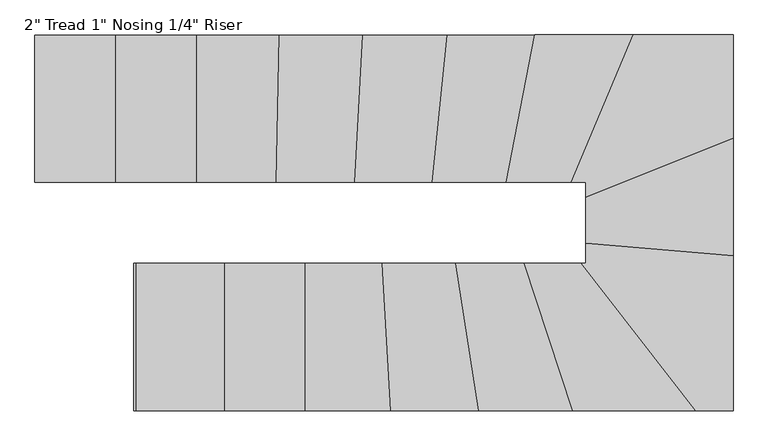
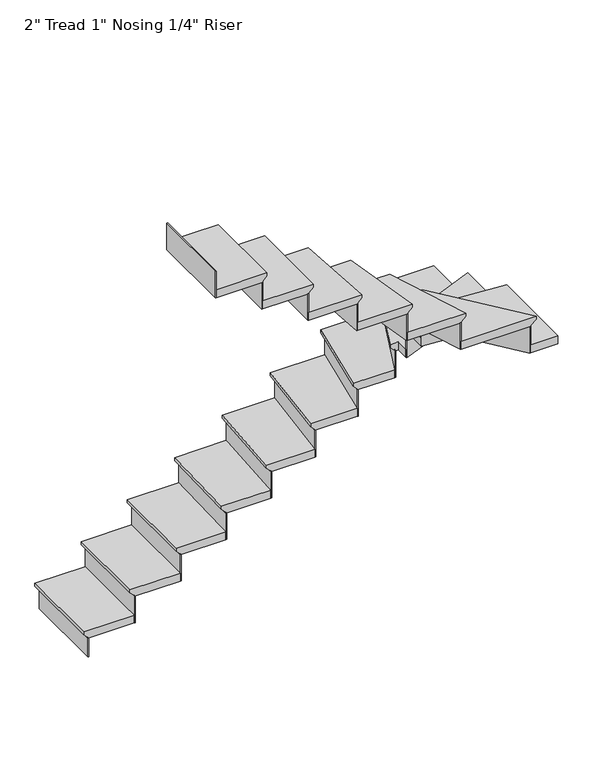
"""IFC4 building model written with IfcOpenShell, lengths in millimetres: stair flight geometry."""

from ifc_helpers import new_model, si_unit, origin, place, context, project, spatial, faceted_brep, source, transform, mapped, element, save


def stair_flight_4e66bfb9(model_context):
    return source(origin(), model_context, "Body", "Brep", [
        faceted_brep([(838.4202681, 2693.877558, 3520.0166667), (838.4202681, 2693.877558, 3539.0666667), (838.4202681, 3202.4524989, 3539.0666667), (838.4202681, 3202.4524989, 3520.0166667), (863.8202681, 2693.877558, 3494.6166667), (863.8202681, 3202.4524989, 3494.6166667), (1143.2202681, 2693.877558, 3539.0666667), (1143.2202681, 3202.4524989, 3539.0666667), (863.8202681, 3202.4524989, 3488.2666667), (1143.2202681, 3202.4524989, 3488.2666667), (1143.2202681, 2693.877558, 3488.2666667), (863.8202681, 2693.877558, 3488.2666667)], [[[0, 1, 2, 3]], [[4, 0, 3, 5]], [[2, 1, 6, 7]], [[8, 9, 10, 11]], [[2, 7, 9, 8, 5, 3]], [[8, 11, 4, 5]], [[6, 1, 0, 4, 11, 10]], [[7, 6, 10, 9]]]),
        faceted_brep([(863.8202681, 2693.877558, 3488.2666667), (863.8202681, 2693.877558, 3369.7333333), (870.1702681, 2693.877558, 3369.7333333), (870.1702681, 2693.877558, 3488.2666667), (863.8202681, 3202.4524989, 3488.2666667), (870.1702681, 3202.4524989, 3488.2666667), (870.1702681, 3202.4524989, 3369.7333333), (863.8202681, 3202.4524989, 3369.7333333)], [[[0, 1, 2, 3]], [[4, 5, 6, 7]], [[1, 0, 4, 7]], [[2, 1, 7, 6]], [[3, 2, 6, 5]], [[0, 3, 5, 4]]]),
        faceted_brep([(1143.2202681, 2693.877558, 3657.6), (1143.2202681, 2693.877558, 3488.2666667), (1149.5702681, 2693.877558, 3488.2666667), (1149.5702681, 2693.877558, 3657.6), (1143.2202681, 3202.4524989, 3657.6), (1149.5702681, 3202.4524989, 3657.6), (1149.5702681, 3202.4524989, 3488.2666667), (1143.2202681, 3202.4524989, 3488.2666667)], [[[0, 1, 2, 3]], [[4, 5, 6, 7]], [[1, 0, 4, 7]], [[2, 1, 7, 6]], [[3, 2, 6, 5]], [[0, 3, 5, 4]]]),
        faceted_brep([(1117.8202681, 3202.4524989, 3708.4), (1117.8202681, 2693.877558, 3708.4), (1422.6202681, 2693.877558, 3708.4), (1422.6202681, 3202.4524989, 3708.4), (1143.2202681, 3202.4524989, 3657.6), (1422.6202681, 3202.4524989, 3657.6), (1422.6202681, 2693.877558, 3657.6), (1143.2202681, 2693.877558, 3657.6), (1143.2202681, 3202.4524989, 3663.95), (1117.8202681, 3202.4524989, 3689.35), (1143.2202681, 2693.877558, 3663.95), (1117.8202681, 2693.877558, 3689.35)], [[[0, 1, 2, 3]], [[4, 5, 6, 7]], [[0, 3, 5, 4, 8, 9]], [[4, 7, 10, 8]], [[2, 1, 11, 10, 7, 6]], [[3, 2, 6, 5]], [[11, 1, 0, 9]], [[10, 11, 9, 8]]]),
        faceted_brep([(1422.6202681, 2693.877558, 3826.9333333), (1422.6202681, 2693.877558, 3657.6), (1428.9702681, 2693.877558, 3657.6), (1428.9702681, 2693.877558, 3826.9333333), (1422.6202681, 3202.4524989, 3826.9333333), (1428.9702681, 3202.4524989, 3826.9333333), (1428.9702681, 3202.4524989, 3657.6), (1422.6202681, 3202.4524989, 3657.6)], [[[0, 1, 2, 3]], [[4, 5, 6, 7]], [[1, 0, 4, 7]], [[2, 1, 7, 6]], [[3, 2, 6, 5]], [[0, 3, 5, 4]]]),
        faceted_brep([(1397.2202681, 3202.4524989, 3877.7333333), (1397.2202681, 2693.877558, 3877.7333333), (1696.6553711, 2693.877558, 3877.7333333), (1707.3964935, 3202.4524989, 3877.7333333), (1422.6202681, 3202.4524989, 3826.9333333), (1707.3964935, 3202.4524989, 3826.9333333), (1696.6553711, 2693.877558, 3826.9333333), (1422.6202681, 2693.877558, 3826.9333333), (1422.6202681, 3202.4524989, 3833.2833333), (1397.2202681, 3202.4524989, 3858.6833333), (1422.6202681, 2693.877558, 3833.2833333), (1397.2202681, 2693.877558, 3858.6833333)], [[[0, 1, 2, 3]], [[4, 5, 6, 7]], [[0, 3, 5, 4, 8, 9]], [[4, 7, 10, 8]], [[2, 1, 11, 10, 7, 6]], [[3, 2, 6, 5]], [[11, 1, 0, 9]], [[10, 11, 9, 8]]]),
        faceted_brep([(1696.6553711, 2693.877558, 3996.2666667), (1696.6553711, 2693.877558, 3826.9333333), (1703.0067872, 2693.877558, 3826.9333333), (1703.0067872, 2693.877558, 3996.2666667), (1707.3964935, 3202.4524989, 3996.2666667), (1713.7479096, 3202.4524989, 3996.2666667), (1713.7479096, 3202.4524989, 3826.9333333), (1707.3964935, 3202.4524989, 3826.9333333)], [[[0, 1, 2, 3]], [[4, 5, 6, 7]], [[1, 0, 4, 7]], [[2, 1, 7, 6]], [[3, 2, 6, 5]], [[0, 3, 5, 4]]]),
        faceted_brep([(1681.9908293, 3202.4524989, 4047.0666667), (1671.2497068, 2693.877558, 4047.0666667), (1968.2389719, 2693.877558, 4047.0666667), (1994.6701229, 3202.4524989, 4047.0666667), (1707.3964935, 3202.4524989, 3996.2666667), (1994.6701229, 3202.4524989, 3996.2666667), (1968.2389719, 2693.877558, 3996.2666667), (1696.6553711, 2693.877558, 3996.2666667), (1707.3964935, 3202.4524989, 4002.6166667), (1681.9908293, 3202.4524989, 4028.0166667), (1696.6553711, 2693.877558, 4002.6166667), (1671.2497068, 2693.877558, 4028.0166667)], [[[0, 1, 2, 3]], [[4, 5, 6, 7]], [[0, 3, 5, 4, 8, 9]], [[4, 7, 10, 8]], [[2, 1, 11, 10, 7, 6]], [[3, 2, 6, 5]], [[11, 1, 0, 9]], [[10, 11, 9, 8]]]),
        faceted_brep([(1968.2389719, 2693.877558, 4165.6), (1968.2389719, 2693.877558, 3996.2666667), (1974.5975418, 2693.877558, 3996.2666667), (1974.5975418, 2693.877558, 4165.6), (1994.6701229, 3202.4524989, 4165.6), (2001.0286928, 3202.4524989, 4165.6), (2001.0286928, 3202.4524989, 3996.2666667), (1994.6701229, 3202.4524989, 3996.2666667)], [[[0, 1, 2, 3]], [[4, 5, 6, 7]], [[1, 0, 4, 7]], [[2, 1, 7, 6]], [[3, 2, 6, 5]], [[0, 3, 5, 4]]]),
        faceted_brep([(1969.2358436, 3202.4524989, 4216.4), (1942.8046925, 2693.877558, 4216.4), (2235.1931673, 2693.877558, 4216.4), (2286.7073051, 3202.4524989, 4216.4), (1994.6701229, 3202.4524989, 4165.6), (2286.7073051, 3202.4524989, 4165.6), (2235.1931673, 2693.877558, 4165.6), (1968.2389719, 2693.877558, 4165.6), (1994.6701229, 3202.4524989, 4171.95), (1969.2358436, 3202.4524989, 4197.35), (1968.2389719, 2693.877558, 4171.95), (1942.8046925, 2693.877558, 4197.35)], [[[0, 1, 2, 3]], [[4, 5, 6, 7]], [[0, 3, 5, 4, 8, 9]], [[4, 7, 10, 8]], [[2, 1, 11, 10, 7, 6]], [[3, 2, 6, 5]], [[11, 1, 0, 9]], [[10, 11, 9, 8]]]),
        faceted_brep([(2235.1931673, 2693.877558, 4334.9333333), (2235.1931673, 2693.877558, 4165.6), (2241.5756594, 2693.877558, 4165.6), (2241.5756594, 2693.877558, 4334.9333333), (2286.7073051, 3202.4524989, 4334.9333333), (2293.0897971, 3202.4524989, 4334.9333333), (2293.0897971, 3202.4524989, 4165.6), (2286.7073051, 3202.4524989, 4165.6)], [[[0, 1, 2, 3]], [[4, 5, 6, 7]], [[1, 0, 4, 7]], [[2, 1, 7, 6]], [[3, 2, 6, 5]], [[0, 3, 5, 4]]]),
        faceted_brep([(2261.1773369, 3202.4524989, 4385.7333333), (2209.6631992, 2693.877558, 4385.7333333), (2491.6737127, 2693.877558, 4385.7333333), (2589.7018996, 3202.4524989, 4385.7333333), (2286.7073051, 3202.4524989, 4334.9333333), (2589.7018996, 3202.4524989, 4334.9333333), (2491.6737127, 2693.877558, 4334.9333333), (2235.1931673, 2693.877558, 4334.9333333), (2286.7073051, 3202.4524989, 4341.2833333), (2261.1773369, 3202.4524989, 4366.6833333), (2235.1931673, 2693.877558, 4341.2833333), (2209.6631992, 2693.877558, 4366.6833333)], [[[0, 1, 2, 3]], [[4, 5, 6, 7]], [[0, 3, 5, 4, 8, 9]], [[4, 7, 10, 8]], [[2, 1, 11, 10, 7, 6]], [[3, 2, 6, 5]], [[11, 1, 0, 9]], [[10, 11, 9, 8]]]),
        faceted_brep([(2491.6737127, 2693.877558, 4504.2666667), (2491.6737127, 2693.877558, 4334.9333333), (2498.1405972, 2693.877558, 4334.9333333), (2498.1405972, 2693.877558, 4504.2666667), (2589.7018996, 3202.4524989, 4504.2666667), (2596.1687841, 3202.4524989, 4504.2666667), (2596.1687841, 3202.4524989, 4334.9333333), (2589.7018996, 3202.4524989, 4334.9333333)], [[[0, 1, 2, 3]], [[4, 5, 6, 7]], [[1, 0, 4, 7]], [[2, 1, 7, 6]], [[3, 2, 6, 5]], [[0, 3, 5, 4]]]),
        faceted_brep([(2563.8343615, 3202.4524989, 4555.0666667), (2465.8061746, 2693.877558, 4555.0666667), (2717.082711, 2693.877558, 4555.0666667), (2931.3822032, 3202.4524989, 4555.0666667), (2589.7018996, 3202.4524989, 4504.2666667), (2931.3822032, 3202.4524989, 4504.2666667), (2717.082711, 2693.877558, 4504.2666667), (2491.6737127, 2693.877558, 4504.2666667), (2589.7018996, 3202.4524989, 4510.6166667), (2563.8343615, 3202.4524989, 4536.0166667), (2491.6737127, 2693.877558, 4510.6166667), (2465.8061746, 2693.877558, 4536.0166667)], [[[0, 1, 2, 3]], [[4, 5, 6, 7]], [[0, 3, 5, 4, 8, 9]], [[4, 7, 10, 8]], [[2, 1, 11, 10, 7, 6]], [[3, 2, 6, 5]], [[11, 1, 0, 9]], [[10, 11, 9, 8]]]),
        faceted_brep([(2717.082711, 2693.877558, 4673.6), (2717.082711, 2693.877558, 4504.2666667), (2723.973426, 2693.877558, 4504.2666667), (2723.973426, 2693.877558, 4673.6), (2931.3822032, 3202.4524989, 4673.6), (2938.2729181, 3202.4524989, 4673.6), (2938.2729181, 3202.4524989, 4504.2666667), (2931.3822032, 3202.4524989, 4504.2666667)], [[[0, 1, 2, 3]], [[4, 5, 6, 7]], [[1, 0, 4, 7]], [[2, 1, 7, 6]], [[3, 2, 6, 5]], [[0, 3, 5, 4]]]),
        faceted_brep([(3247.982332, 2818.4435318, 4724.4), (3247.982332, 3202.4524989, 4724.4), (2903.8193433, 3202.4524989, 4724.4), (2689.5198512, 2693.877558, 4724.4), (2739.4073911, 2693.877558, 4724.4), (2739.4073911, 2614.5975609, 4724.4), (3247.982332, 3202.4524989, 4673.6), (3247.982332, 2818.4435318, 4673.6), (2739.4073911, 2614.5975609, 4673.6), (2739.4073911, 2693.877558, 4673.6), (2717.082711, 2693.877558, 4673.6), (2931.3822032, 3202.4524989, 4673.6), (2717.082711, 2693.877558, 4679.95), (2931.3822032, 3202.4524989, 4679.95), (2689.5198512, 2693.877558, 4705.35), (2903.8193433, 3202.4524989, 4705.35)], [[[0, 1, 2, 3, 4, 5]], [[6, 7, 8, 9, 10, 11]], [[1, 0, 7, 6]], [[11, 10, 12, 13]], [[5, 4, 9, 8]], [[0, 5, 8, 7]], [[14, 3, 2, 15]], [[12, 14, 15, 13]], [[4, 3, 14, 12, 10, 9]], [[2, 1, 6, 11, 13, 15]]]),
        faceted_brep([(2739.4073911, 2614.5975609, 4842.9333333), (2739.4073911, 2614.5975609, 4673.6), (2739.4073911, 2607.7564709, 4673.6), (2739.4073911, 2607.7564709, 4842.9333333), (3247.982332, 2818.4435318, 4842.9333333), (3247.982332, 2811.6024418, 4842.9333333), (3247.982332, 2811.6024418, 4673.6), (3247.982332, 2818.4435318, 4673.6)], [[[0, 1, 2, 3]], [[4, 5, 6, 7]], [[1, 0, 4, 7]], [[2, 1, 7, 6]], [[3, 2, 6, 5]], [[0, 3, 5, 4]]]),
        faceted_brep([(3247.982332, 2845.807892, 4893.7333333), (2739.4073911, 2641.9619211, 4893.7333333), (2739.4073911, 2458.7583414, 4893.7333333), (3247.982332, 2415.6151582, 4893.7333333), (3247.982332, 2818.4435318, 4842.9333333), (3247.982332, 2415.6151582, 4842.9333333), (2739.4073911, 2458.7583414, 4842.9333333), (2739.4073911, 2614.5975609, 4842.9333333), (3247.982332, 2818.4435318, 4849.2833333), (3247.982332, 2845.807892, 4874.6833333), (2739.4073911, 2614.5975609, 4849.2833333), (2739.4073911, 2641.9619211, 4874.6833333)], [[[0, 1, 2, 3]], [[4, 5, 6, 7]], [[0, 3, 5, 4, 8, 9]], [[4, 7, 10, 8]], [[2, 1, 11, 10, 7, 6]], [[3, 2, 6, 5]], [[11, 1, 0, 9]], [[10, 11, 9, 8]]]),
        faceted_brep([(2739.4073911, 2458.7583414, 5012.2666667), (2739.4073911, 2458.7583414, 4842.9333333), (2739.4073911, 2452.3855338, 4842.9333333), (2739.4073911, 2452.3855338, 5012.2666667), (3247.982332, 2415.6151582, 5012.2666667), (3247.982332, 2409.2423506, 5012.2666667), (3247.982332, 2409.2423506, 4842.9333333), (3247.982332, 2415.6151582, 4842.9333333)], [[[0, 1, 2, 3]], [[4, 5, 6, 7]], [[1, 0, 4, 7]], [[2, 1, 7, 6]], [[3, 2, 6, 5]], [[0, 3, 5, 4]]]),
        faceted_brep([(3085.5772675, 1905.9026171, 5063.0666667), (3247.982332, 1905.9026171, 5063.0666667), (3247.982332, 2441.1063885, 5063.0666667), (2739.4073911, 2484.2495716, 5063.0666667), (2739.4073911, 2414.477558, 5063.0666667), (2689.4386829, 2414.477558, 5063.0666667), (3247.982332, 1905.9026171, 5012.2666667), (3085.5772675, 1905.9026171, 5012.2666667), (2689.4386829, 2414.477558, 5012.2666667), (2739.4073911, 2414.477558, 5012.2666667), (2739.4073911, 2458.7583414, 5012.2666667), (3247.982332, 2415.6151582, 5012.2666667), (2739.4073911, 2458.7583414, 5018.6166667), (3247.982332, 2415.6151582, 5018.6166667), (2739.4073911, 2484.2495716, 5044.0166667), (3247.982332, 2441.1063885, 5044.0166667)], [[[0, 1, 2, 3, 4, 5]], [[6, 7, 8, 9, 10, 11]], [[1, 0, 7, 6]], [[11, 10, 12, 13]], [[4, 3, 14, 12, 10, 9]], [[5, 4, 9, 8]], [[0, 5, 8, 7]], [[14, 3, 2, 15]], [[12, 14, 15, 13]], [[2, 1, 6, 11, 13, 15]]]),
        faceted_brep([(2689.4386829, 2414.477558, 5181.6), (2689.4386829, 2414.477558, 5012.2666667), (2681.3896615, 2414.477558, 5012.2666667), (2681.3896615, 2414.477558, 5181.6), (3085.5772675, 1905.9026171, 5181.6), (3077.5282461, 1905.9026171, 5181.6), (3077.5282461, 1905.9026171, 5012.2666667), (3085.5772675, 1905.9026171, 5012.2666667)], [[[0, 1, 2, 3]], [[4, 5, 6, 7]], [[1, 0, 4, 7]], [[2, 1, 7, 6]], [[3, 2, 6, 5]], [[0, 3, 5, 4]]]),
        faceted_brep([(3117.7733531, 1905.9026171, 5232.4), (2721.6347685, 2414.477558, 5232.4), (2498.169104, 2414.477558, 5232.4), (2665.6971357, 1905.9026171, 5232.4), (3085.5772675, 1905.9026171, 5181.6), (2665.6971357, 1905.9026171, 5181.6), (2498.169104, 2414.477558, 5181.6), (2689.4386829, 2414.477558, 5181.6), (3085.5772675, 1905.9026171, 5187.95), (3117.7733531, 1905.9026171, 5213.35), (2689.4386829, 2414.477558, 5187.95), (2721.6347685, 2414.477558, 5213.35)], [[[0, 1, 2, 3]], [[4, 5, 6, 7]], [[0, 3, 5, 4, 8, 9]], [[4, 7, 10, 8]], [[2, 1, 11, 10, 7, 6]], [[3, 2, 6, 5]], [[11, 1, 0, 9]], [[10, 11, 9, 8]]]),
        faceted_brep([(2498.169104, 2414.477558, 5350.9333333), (2498.169104, 2414.477558, 5181.6), (2491.4834592, 2414.477558, 5181.6), (2491.4834592, 2414.477558, 5350.9333333), (2665.6971357, 1905.9026171, 5350.9333333), (2659.0114908, 1905.9026171, 5350.9333333), (2659.0114908, 1905.9026171, 5181.6), (2665.6971357, 1905.9026171, 5181.6)], [[[0, 1, 2, 3]], [[4, 5, 6, 7]], [[1, 0, 4, 7]], [[2, 1, 7, 6]], [[3, 2, 6, 5]], [[0, 3, 5, 4]]]),
        faceted_brep([(2692.4397151, 1905.9026171, 5401.7333333), (2524.9116834, 2414.477558, 5401.7333333), (2264.2527614, 2414.477558, 5401.7333333), (2342.8948816, 1905.9026171, 5401.7333333), (2665.6971357, 1905.9026171, 5350.9333333), (2342.8948816, 1905.9026171, 5350.9333333), (2264.2527614, 2414.477558, 5350.9333333), (2498.169104, 2414.477558, 5350.9333333), (2665.6971357, 1905.9026171, 5357.2833333), (2692.4397151, 1905.9026171, 5382.6833333), (2498.169104, 2414.477558, 5357.2833333), (2524.9116834, 2414.477558, 5382.6833333)], [[[0, 1, 2, 3]], [[4, 5, 6, 7]], [[0, 3, 5, 4, 8, 9]], [[4, 7, 10, 8]], [[2, 1, 11, 10, 7, 6]], [[3, 2, 6, 5]], [[11, 1, 0, 9]], [[10, 11, 9, 8]]]),
        faceted_brep([(2264.2527614, 2414.477558, 5520.2666667), (2264.2527614, 2414.477558, 5350.9333333), (2257.827292, 2414.477558, 5350.9333333), (2257.827292, 2414.477558, 5520.2666667), (2342.8948816, 1905.9026171, 5520.2666667), (2336.4694122, 1905.9026171, 5520.2666667), (2336.4694122, 1905.9026171, 5350.9333333), (2342.8948816, 1905.9026171, 5350.9333333)], [[[0, 1, 2, 3]], [[4, 5, 6, 7]], [[1, 0, 4, 7]], [[2, 1, 7, 6]], [[3, 2, 6, 5]], [[0, 3, 5, 4]]]),
        faceted_brep([(2368.5967594, 1905.9026171, 5571.0666667), (2289.9546392, 2414.477558, 5571.0666667), (2009.2587296, 2414.477558, 5571.0666667), (2039.6023306, 1905.9026171, 5571.0666667), (2342.8948816, 1905.9026171, 5520.2666667), (2039.6023306, 1905.9026171, 5520.2666667), (2009.2587296, 2414.477558, 5520.2666667), (2264.2527614, 2414.477558, 5520.2666667), (2342.8948816, 1905.9026171, 5526.6166667), (2368.5967594, 1905.9026171, 5552.0166667), (2264.2527614, 2414.477558, 5526.6166667), (2289.9546392, 2414.477558, 5552.0166667)], [[[0, 1, 2, 3]], [[4, 5, 6, 7]], [[0, 3, 5, 4, 8, 9]], [[4, 7, 10, 8]], [[2, 1, 11, 10, 7, 6]], [[3, 2, 6, 5]], [[11, 1, 0, 9]], [[10, 11, 9, 8]]]),
        faceted_brep([(2009.2587296, 2414.477558, 5689.6), (2009.2587296, 2414.477558, 5520.2666667), (2002.8974373, 2414.477558, 5520.2666667), (2002.8974373, 2414.477558, 5689.6), (2039.6023306, 1905.9026171, 5689.6), (2033.2410383, 1905.9026171, 5689.6), (2033.2410383, 1905.9026171, 5520.2666667), (2039.6023306, 1905.9026171, 5520.2666667)], [[[0, 1, 2, 3]], [[4, 5, 6, 7]], [[1, 0, 4, 7]], [[2, 1, 7, 6]], [[3, 2, 6, 5]], [[0, 3, 5, 4]]]),
        faceted_brep([(2065.0474997, 1905.9026171, 5740.4), (2034.7038988, 2414.477558, 5740.4), (1745.0756993, 2414.477558, 5740.4), (1745.0756993, 1905.9026171, 5740.4), (2039.6023306, 1905.9026171, 5689.6), (1745.0756993, 1905.9026171, 5689.6), (1745.0756993, 2414.477558, 5689.6), (2009.2587296, 2414.477558, 5689.6), (2039.6023306, 1905.9026171, 5695.95), (2065.0474997, 1905.9026171, 5721.35), (2009.2587296, 2414.477558, 5695.95), (2034.7038988, 2414.477558, 5721.35)], [[[0, 1, 2, 3]], [[4, 5, 6, 7]], [[0, 3, 5, 4, 8, 9]], [[4, 7, 10, 8]], [[2, 1, 11, 10, 7, 6]], [[3, 2, 6, 5]], [[11, 1, 0, 9]], [[10, 11, 9, 8]]]),
        faceted_brep([(1745.0756993, 2414.477558, 5858.9333333), (1745.0756993, 2414.477558, 5689.6), (1738.7256993, 2414.477558, 5689.6), (1738.7256993, 2414.477558, 5858.9333333), (1745.0756993, 1905.9026171, 5858.9333333), (1738.7256993, 1905.9026171, 5858.9333333), (1738.7256993, 1905.9026171, 5689.6), (1745.0756993, 1905.9026171, 5689.6)], [[[0, 1, 2, 3]], [[4, 5, 6, 7]], [[1, 0, 4, 7]], [[2, 1, 7, 6]], [[3, 2, 6, 5]], [[0, 3, 5, 4]]]),
        faceted_brep([(1770.4756993, 1905.9026171, 5909.7333333), (1770.4756993, 2414.477558, 5909.7333333), (1465.6756993, 2414.477558, 5909.7333333), (1465.6756993, 1905.9026171, 5909.7333333), (1745.0756993, 1905.9026171, 5858.9333333), (1465.6756993, 1905.9026171, 5858.9333333), (1465.6756993, 2414.477558, 5858.9333333), (1745.0756993, 2414.477558, 5858.9333333), (1745.0756993, 1905.9026171, 5865.2833333), (1770.4756993, 1905.9026171, 5890.6833333), (1745.0756993, 2414.477558, 5865.2833333), (1770.4756993, 2414.477558, 5890.6833333)], [[[0, 1, 2, 3]], [[4, 5, 6, 7]], [[0, 3, 5, 4, 8, 9]], [[4, 7, 10, 8]], [[2, 1, 11, 10, 7, 6]], [[3, 2, 6, 5]], [[11, 1, 0, 9]], [[10, 11, 9, 8]]]),
        faceted_brep([(1465.6756993, 2414.477558, 6028.2666667), (1465.6756993, 2414.477558, 5858.9333333), (1459.3256993, 2414.477558, 5858.9333333), (1459.3256993, 2414.477558, 6028.2666667), (1465.6756993, 1905.9026171, 6028.2666667), (1459.3256993, 1905.9026171, 6028.2666667), (1459.3256993, 1905.9026171, 5858.9333333), (1465.6756993, 1905.9026171, 5858.9333333)], [[[0, 1, 2, 3]], [[4, 5, 6, 7]], [[1, 0, 4, 7]], [[2, 1, 7, 6]], [[3, 2, 6, 5]], [[0, 3, 5, 4]]]),
        faceted_brep([(1186.2756993, 2414.477558, 6197.6), (1186.2756993, 2414.477558, 6028.2666667), (1179.9256993, 2414.477558, 6028.2666667), (1179.9256993, 2414.477558, 6197.6), (1186.2756993, 1905.9026171, 6197.6), (1179.9256993, 1905.9026171, 6197.6), (1179.9256993, 1905.9026171, 6028.2666667), (1186.2756993, 1905.9026171, 6028.2666667)], [[[0, 1, 2, 3]], [[4, 5, 6, 7]], [[1, 0, 4, 7]], [[2, 1, 7, 6]], [[3, 2, 6, 5]], [[0, 3, 5, 4]]]),
        faceted_brep([(1491.0756993, 1905.9026171, 6079.0666667), (1491.0756993, 2414.477558, 6079.0666667), (1186.2756993, 2414.477558, 6079.0666667), (1186.2756993, 1905.9026171, 6079.0666667), (1465.6756993, 1905.9026171, 6028.2666667), (1186.2756993, 1905.9026171, 6028.2666667), (1186.2756993, 2414.477558, 6028.2666667), (1465.6756993, 2414.477558, 6028.2666667), (1465.6756993, 1905.9026171, 6034.6166667), (1491.0756993, 1905.9026171, 6060.0166667), (1465.6756993, 2414.477558, 6034.6166667), (1491.0756993, 2414.477558, 6060.0166667)], [[[0, 1, 2, 3]], [[4, 5, 6, 7]], [[0, 3, 5, 4, 8, 9]], [[4, 7, 10, 8]], [[2, 1, 11, 10, 7, 6]], [[3, 2, 6, 5]], [[11, 1, 0, 9]], [[10, 11, 9, 8]]]),
    ])


if __name__ == "__main__":
    model = new_model("IFC4")
    model_context = context("Model", 3, world=origin())
    ifc_project = project(units=[si_unit("LENGTHUNIT", "METRE", prefix="MILLI")], contexts=[model_context])
    site = spatial("IfcSite", under=ifc_project)
    building = spatial("IfcBuilding", under=site)
    placement = place(None, origin())
    stair_flight_shape = stair_flight_4e66bfb9(model_context)
    element("IfcStairFlight", 1, ObjectType="2\" Tread 1\" Nosing 1/4\" Riser", at=placement, inside=building, context=model_context, shape_type="MappedRepresentation", body=[
        mapped(stair_flight_shape, transform((0.0, 0.0, 0.0), x_axis=(1.0, 0.0, 0.0), y_axis=(0.0, 1.0, 0.0), z_axis=(0.0, 0.0, 1.0))),
    ])
    save(model, "model.ifc")
